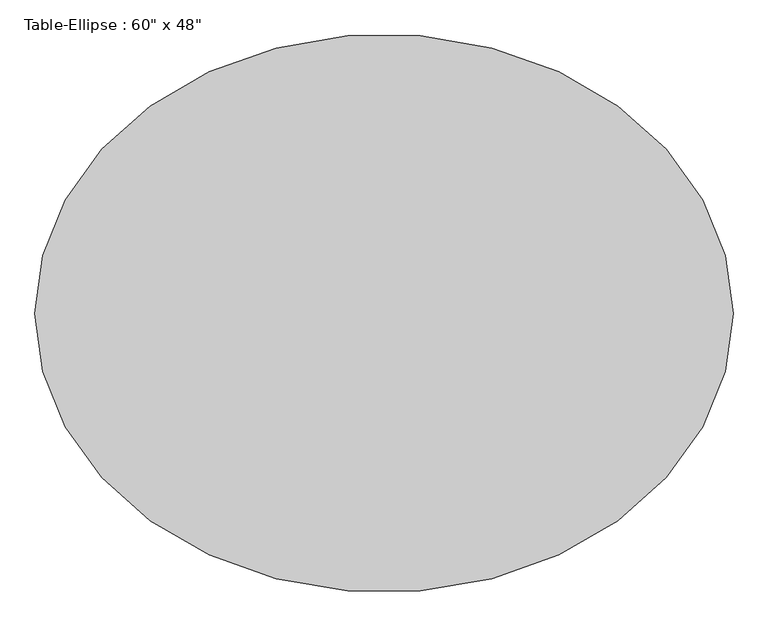
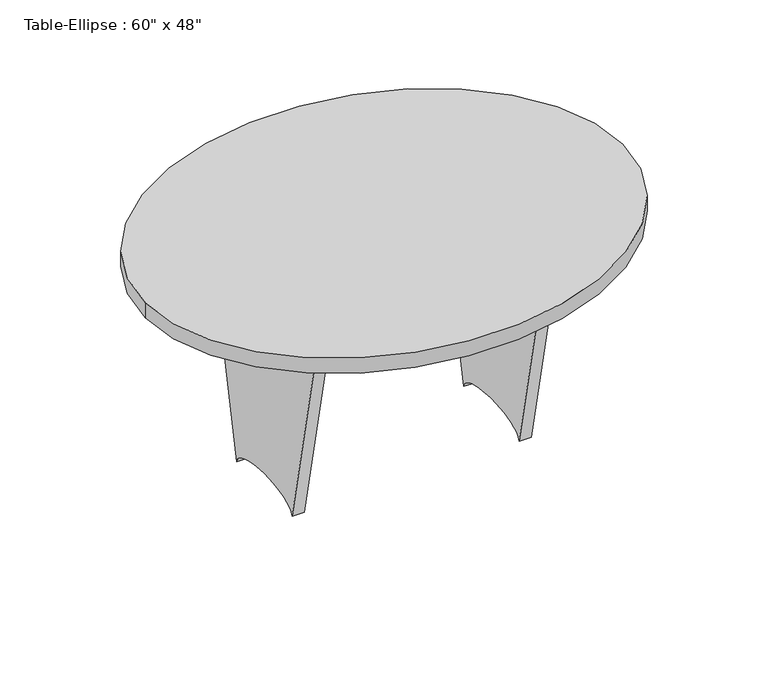
"""IFC4 building model written with IfcOpenShell, lengths in millimetres: furniture geometry."""

from ifc_helpers import new_model, si_unit, point, frame, origin, place, context, project, spatial, ellipse_curve, trimmed, source, transform, mapped, element, save
from ifc_brep_helpers import plane_surface, extruded_surface, advanced_brep


def furniture_743965d2(model_context):
    return source(origin(), model_context, "Body", "AdvancedBrep", [
        advanced_brep(
        [(-342.9, 19.05, 711.2), (342.9, 19.05, 711.2), (342.9, 19.05, 474.1333333), (-342.9, 19.05, 474.1333333), (-342.9, -19.05, 711.2), (-342.9, -19.05, 474.1333333), (342.9, -19.05, 474.1333333), (342.9, -19.05, 711.2)],
        [
            (0, 1),
            (1, 2),
            (2, 3, ellipse_curve(frame((0.0, 19.05, 474.1333333), z_axis=(0.0, -1.0, 0.0), x_axis=(1.0, 0.0, 0.0)), 342.9, 101.6)),
            (3, 0),
            (4, 5),
            (5, 6, ellipse_curve(frame((0.0, -19.05, 474.1333333), z_axis=(0.0, 1.0, 0.0), x_axis=(1.0, 0.0, 0.0)), 342.9, 101.6)),
            (6, 7),
            (7, 4),
            (0, 4),
            (7, 1),
            (6, 2),
            (5, 3),
        ],
        [
            plane_surface(frame((-342.9, 19.05, 711.2), z_axis=(0.0, 1.0, 0.0), x_axis=(1.0, 0.0, 0.0))),
            plane_surface(frame((-342.9, -19.05, 711.2), z_axis=(0.0, -1.0, 0.0), x_axis=(-1.0, 0.0, 0.0))),
            plane_surface(frame((-342.9, 19.05, 711.2), z_axis=(0.0, 0.0, 1.0), x_axis=(0.0, -1.0, 0.0))),
            plane_surface(frame((342.9, 19.05, 711.2), z_axis=(1.0, 0.0, 0.0), x_axis=(0.0, -1.0, 0.0))),
            extruded_surface(trimmed(ellipse_curve(frame((0.0, -57.15, 474.1333333), z_axis=(0.0, -1.0, 0.0), x_axis=(1.0, 0.0, 0.0)), 342.9, 101.6), [point((342.9, -57.15, 474.1333333))], [point((-342.9, -57.15, 474.1333333))], True, "CARTESIAN"), (0.0, 38.099999999999994, 0.0), 38.099999999999994),
            plane_surface(frame((-342.9, 19.05, 474.1333333), z_axis=(-1.0, 0.0, 0.0), x_axis=(0.0, -1.0, 0.0))),
        ],
        [
            (0, [[1, 2, 3, 4]]),
            (1, [[5, 6, 7, 8]]),
            (2, [[-1, 9, -8, 10]]),
            (3, [[-2, -10, -7, 11]]),
            (4, [[-3, -11, -6, 12]]),
            (5, [[-4, -12, -5, -9]]),
        ],
    ),
        advanced_brep(
        [(381.0, 304.8, 711.2), (381.0, -304.8, 711.2), (381.0, -152.4, 0.0), (381.0, 152.4, 0.0), (342.9, 304.8, 711.2), (342.9, 152.4, 0.0), (342.9, -152.4, 0.0), (342.9, -304.8, 711.2)],
        [
            (0, 1),
            (1, 2),
            (2, 3, ellipse_curve(frame((381.0, 0.0, 0.0), z_axis=(-1.0, 0.0, 0.0), x_axis=(0.0, 1.0, 0.0)), 152.4, 50.8)),
            (3, 0),
            (4, 5),
            (5, 6, ellipse_curve(frame((342.9, 0.0, 0.0), z_axis=(1.0, 0.0, 0.0), x_axis=(0.0, 1.0, 0.0)), 152.4, 50.8)),
            (6, 7),
            (7, 4),
            (0, 4),
            (7, 1),
            (6, 2),
            (5, 3),
        ],
        [
            plane_surface(frame((381.0, -304.8, 711.2), z_axis=(1.0, 0.0, 0.0), x_axis=(0.0, -1.0, 0.0))),
            plane_surface(frame((342.9, -304.8, 711.2), z_axis=(-1.0, 0.0, 0.0), x_axis=(0.0, 1.0, 0.0))),
            plane_surface(frame((381.0, 304.8, 711.2), z_axis=(0.0, 0.0, 1.0), x_axis=(-1.0, 0.0, 0.0))),
            plane_surface(frame((381.0, -304.8, 711.2), z_axis=(0.0, -0.9778024140774091, -0.2095290887308754), x_axis=(-1.0, 0.0, 0.0))),
            extruded_surface(trimmed(ellipse_curve(frame((304.8, 0.0, 0.0), z_axis=(-1.0, 0.0, 0.0), x_axis=(0.0, 1.0, 0.0)), 152.4, 50.8), [point((304.8, -152.4, 0.0))], [point((304.8, 152.4, 0.0))], True, "CARTESIAN"), (38.099999999999966, 0.0, 0.0), 38.099999999999966),
            plane_surface(frame((381.0, 152.4, 0.0), z_axis=(0.0, 0.977802414077412, -0.2095290887308621), x_axis=(-1.0, 0.0, 0.0))),
        ],
        [
            (0, [[1, 2, 3, 4]]),
            (1, [[5, 6, 7, 8]]),
            (2, [[-1, 9, -8, 10]]),
            (3, [[-2, -10, -7, 11]]),
            (4, [[-3, -11, -6, 12]]),
            (5, [[-4, -12, -5, -9]]),
        ],
    ),
        advanced_brep(
        [(-342.9, 304.8, 711.2), (-342.9, -304.8, 711.2), (-342.9, -152.4, 0.0), (-342.9, 152.4, 0.0), (-381.0, 304.8, 711.2), (-381.0, 152.4, 0.0), (-381.0, -152.4, 0.0), (-381.0, -304.8, 711.2)],
        [
            (0, 1),
            (1, 2),
            (2, 3, ellipse_curve(frame((-342.9, 0.0, 0.0), z_axis=(-1.0, 0.0, 0.0), x_axis=(0.0, 1.0, 0.0)), 152.4, 50.8)),
            (3, 0),
            (4, 5),
            (5, 6, ellipse_curve(frame((-381.0, 0.0, 0.0), z_axis=(1.0, 0.0, 0.0), x_axis=(0.0, 1.0, 0.0)), 152.4, 50.8)),
            (6, 7),
            (7, 4),
            (0, 4),
            (7, 1),
            (6, 2),
            (5, 3),
        ],
        [
            plane_surface(frame((-342.9, -304.8, 711.2), z_axis=(1.0, 0.0, 0.0), x_axis=(0.0, -1.0, 0.0))),
            plane_surface(frame((-381.0, -304.8, 711.2), z_axis=(-1.0, 0.0, 0.0), x_axis=(0.0, 1.0, 0.0))),
            plane_surface(frame((-342.9, 304.8, 711.2), z_axis=(0.0, 0.0, 1.0), x_axis=(-1.0, 0.0, 0.0))),
            plane_surface(frame((-342.9, -304.8, 711.2), z_axis=(0.0, -0.9778024140774088, -0.2095290887308767), x_axis=(-1.0, 0.0, 0.0))),
            extruded_surface(trimmed(ellipse_curve(frame((-419.1, 0.0, 0.0), z_axis=(-1.0, 0.0, 0.0), x_axis=(0.0, 1.0, 0.0)), 152.4, 50.8), [point((-419.1, -152.4, 0.0))], [point((-419.1, 152.4, 0.0))], True, "CARTESIAN"), (38.10000000000002, 0.0, 0.0), 38.10000000000002),
            plane_surface(frame((-342.9, 152.4, 0.0), z_axis=(0.0, 0.9778024140774109, -0.2095290887308677), x_axis=(-1.0, 0.0, 0.0))),
        ],
        [
            (0, [[1, 2, 3, 4]]),
            (1, [[5, 6, 7, 8]]),
            (2, [[-1, 9, -8, 10]]),
            (3, [[-2, -10, -7, 11]]),
            (4, [[-3, -11, -6, 12]]),
            (5, [[-4, -12, -5, -9]]),
        ],
    ),
        advanced_brep(
        [(-762.0, 0.0, 762.0), (762.0, 0.0, 762.0), (-762.0, 0.0, 711.2), (762.0, 0.0, 711.2)],
        [
            (0, 1, ellipse_curve(frame((0.0, 0.0, 762.0), z_axis=(0.0, 0.0, 1.0), x_axis=(1.0, 0.0, 0.0)), 762.0, 609.6)),
            (1, 0, ellipse_curve(frame((0.0, 0.0, 762.0), z_axis=(0.0, 0.0, 1.0), x_axis=(1.0, 0.0, 0.0)), 762.0, 609.6)),
            (2, 3, ellipse_curve(frame((0.0, 0.0, 711.2), z_axis=(0.0, 0.0, -1.0), x_axis=(1.0, 0.0, 0.0)), 762.0, 609.6)),
            (3, 2, ellipse_curve(frame((0.0, 0.0, 711.2), z_axis=(0.0, 0.0, -1.0), x_axis=(1.0, 0.0, 0.0)), 762.0, 609.6)),
            (0, 2),
            (3, 1),
        ],
        [
            plane_surface(frame((762.0, 0.0, 762.0), z_axis=(0.0, 0.0, 1.0), x_axis=(0.0, 1.0, 0.0))),
            plane_surface(frame((762.0, 0.0, 711.2), z_axis=(0.0, 0.0, -1.0), x_axis=(0.0, -1.0, 0.0))),
            extruded_surface(trimmed(ellipse_curve(frame((0.0, 0.0, 660.4), z_axis=(0.0, 0.0, 1.0), x_axis=(1.0, 0.0, 0.0)), 762.0, 609.6), [point((-762.0, 0.0, 660.4))], [point((762.0, 0.0, 660.4))], True, "CARTESIAN"), (0.0, 0.0, 50.80000000000007), 50.80000000000007),
            extruded_surface(trimmed(ellipse_curve(frame((0.0, 0.0, 660.4), z_axis=(0.0, 0.0, 1.0), x_axis=(1.0, 0.0, 0.0)), 762.0, 609.6), [point((762.0, 0.0, 660.4))], [point((-762.0, 0.0, 660.4))], True, "CARTESIAN"), (0.0, 0.0, 50.80000000000007), 50.80000000000007),
        ],
        [
            (0, [[1, 2]]),
            (1, [[3, 4]]),
            (2, [[-1, 5, -4, 6]]),
            (3, [[-2, -6, -3, -5]]),
        ],
    ),
    ])


if __name__ == "__main__":
    model = new_model("IFC4")
    model_context = context("Model", 3, world=origin())
    ifc_project = project(units=[si_unit("LENGTHUNIT", "METRE", prefix="MILLI")], contexts=[model_context])
    site = spatial("IfcSite", under=ifc_project)
    building = spatial("IfcBuilding", under=site)
    placement = place(None, origin())
    furniture_shape = furniture_743965d2(model_context)
    element("IfcFurniture", 1, ObjectType="Table-Ellipse : 60\" x 48\"", at=placement, inside=building, context=model_context, shape_type="MappedRepresentation", body=[
        mapped(furniture_shape, transform((0.0, 0.0, 0.0), x_axis=(1.0, 0.0, 0.0), y_axis=(0.0, 1.0, 0.0), z_axis=(0.0, 0.0, 1.0))),
    ])
    save(model, "model.ifc")

# Revit data of these elements
# Type "Table-Ellipse : 60\" x 48\""
#   Assembly Code = "E2020200"
#   Half Width = 2' - 0"
#   Half Length = 2' - 6"
#   Height = 2' - 6"
#   Length = 5' - 0"
#   Width = 4' - 0"
#   Base Material = Birch
#   Top Material = Birch
#   Default Elevation = 0
# Element 1 (IfcFurniture, "Table-Ellipse : 60\" x 48\"")
#   Materials on its faces: "Birch"
# Materials
#   "Birch": class "Wood", colour RGB 210 159 95, transparency 0, Description = "Betula Alleghaniensis", Cost = 0
